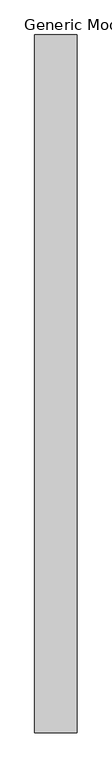
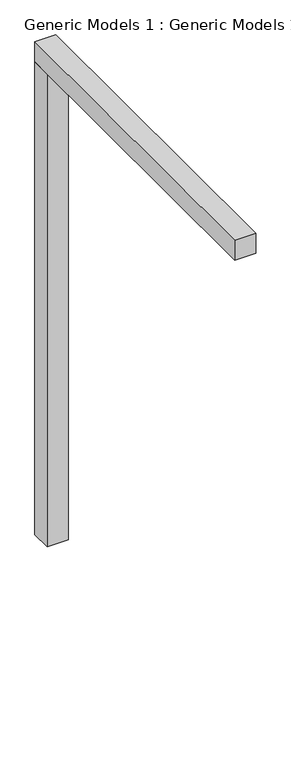
"""IFC4 building model written with IfcOpenShell, lengths in millimetres: proxy geometry, Generic Models 1 : Generic Models 1."""

from ifc_helpers import new_model, si_unit, frame, origin, place, context, project, spatial, polyline, outline, extrude, source, transform, mapped, element, save


def generic_models_1_generic_models_1_001e7bd1(model_context):
    return source(origin(), model_context, "Body", "SweptSolid", [
        extrude(outline(polyline([(-1950.9656154, 7090.2500875), (-1950.9656154, 2072.4507558), (-2255.7656154, 2072.4507558), (-2255.7656154, 7090.2500875), (-1950.9656154, 7090.2500875)])), frame((0.0, 0.0, 8839.2), z_axis=(0.0, 0.0, 1.0), x_axis=(1.0, 0.0, 0.0)), (0.0, 0.0, 1.0), 304.8),
        extrude(outline(polyline([(-1950.9656154, 7090.2500875), (-1950.9656154, 6785.4500875), (-2255.7656154, 6785.4500875), (-2255.7656154, 7090.2500875), (-1950.9656154, 7090.2500875)])), frame((0.0, 0.0, 1585.0545123), z_axis=(0.0, 0.0, 1.0), x_axis=(1.0, 0.0, 0.0)), (0.0, 0.0, 1.0), 7253.0500734),
    ])


if __name__ == "__main__":
    model = new_model("IFC4")
    model_context = context("Model", 3, world=origin())
    ifc_project = project(units=[si_unit("LENGTHUNIT", "METRE", prefix="MILLI")], contexts=[model_context])
    site = spatial("IfcSite", under=ifc_project)
    building = spatial("IfcBuilding", under=site)
    placement = place(None, origin())
    generic_models_1_generic_models_1_shape = generic_models_1_generic_models_1_001e7bd1(model_context)
    element("IfcBuildingElementProxy", 1, Name="Generic Models 1 : Generic Models 1", ObjectType="Generic Models 1 : Generic Models 1", at=placement, inside=building, context=model_context, shape_type="MappedRepresentation", body=[
        mapped(generic_models_1_generic_models_1_shape, transform((0.0, 0.0, 0.0), x_axis=(1.0, 0.0, 0.0), y_axis=(0.0, 1.0, 0.0), z_axis=(0.0, 0.0, 1.0))),
    ])
    save(model, "model.ifc")

# Revit data of these elements
# Element 1 (IfcBuildingElementProxy, "Generic Models 1 : Generic Models 1")
#   Materials on its faces: "LIGHT BEIGE"
# Materials
#   "LIGHT BEIGE": class "Generic", colour RGB 120 120 120, transparency 0, Cost = 0
